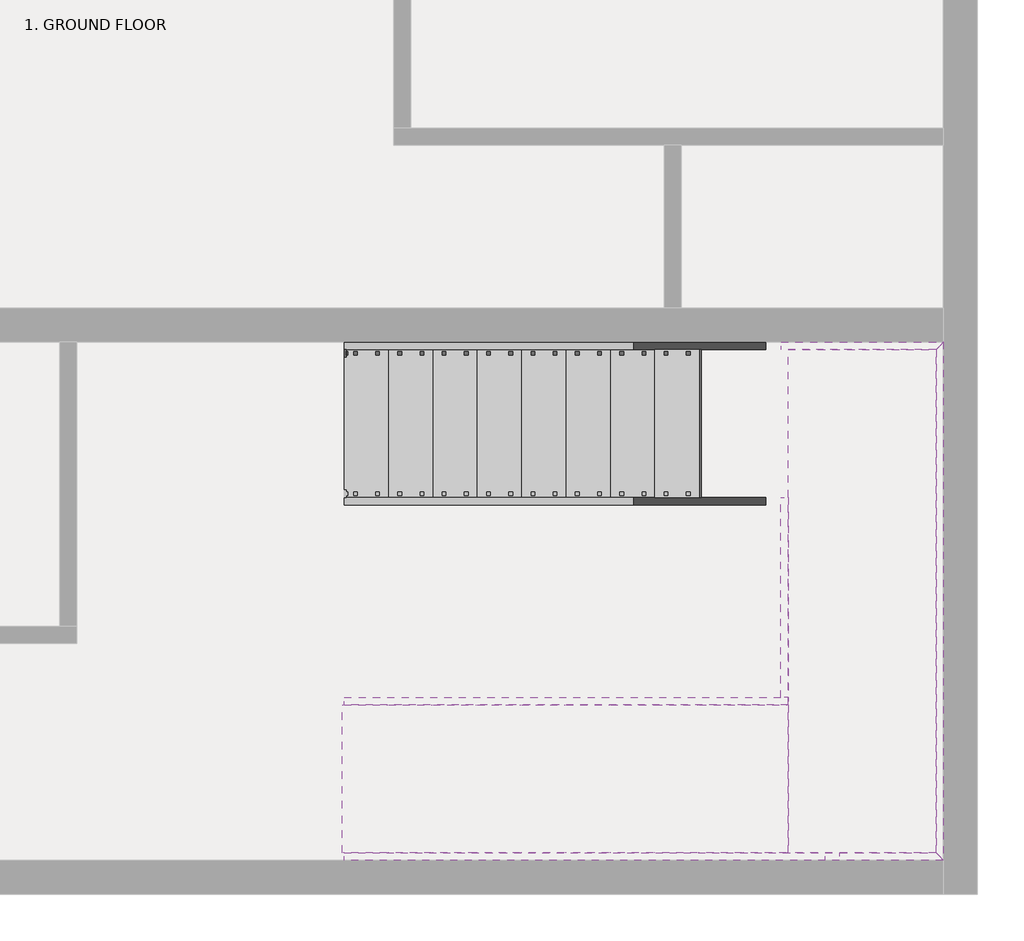
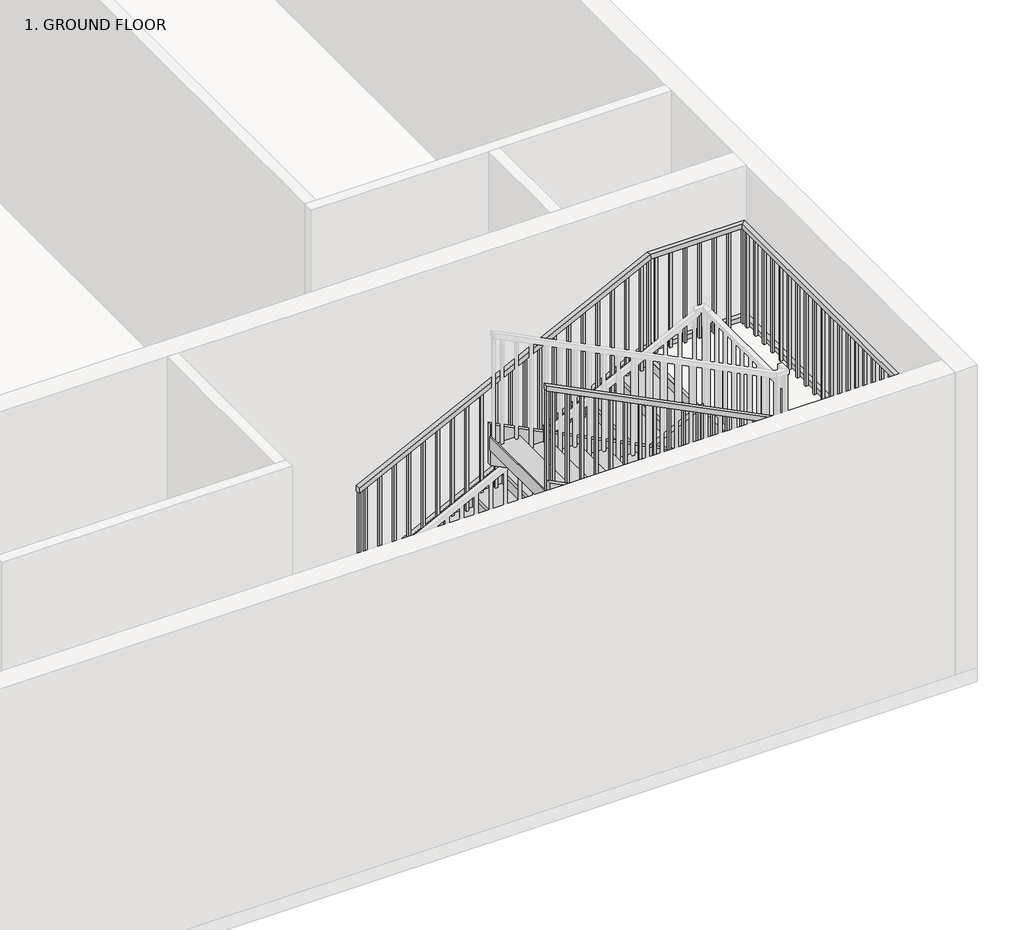
# One storey, part 2 of 2: 8 members, 2 stair flights, 1 railing, 1 slab.
"""IFC4 building model written with IfcOpenShell, lengths in millimetres."""

from ifc_helpers import new_model, si_unit, frame, origin, place, context, project, spatial, polyline, outline, extrude, faceted_brep, transform, mapped, element, save
from components import non_monolithic_landing_146c630b, stair_flight_50mm_tread_13mm_riser_b7d47cc6, stair_flight_50mm_tread_13mm_riser_afbce6aa

model = new_model("IFC4")

# Units and contexts
model_context = context("Model", 3, world=origin())
ifc_project = project(units=[si_unit("LENGTHUNIT", "METRE", prefix="MILLI")], contexts=[model_context])

# Site, building, storey
site = spatial("IfcSite", under=ifc_project)
building = spatial("IfcBuilding", under=site)
storey = spatial("IfcBuildingStorey", under=building, Name="1. GROUND FLOOR", Elevation=0.0)

# Members
placement = place(None, origin())
element("IfcMember", 1, ObjectType="Stringer - 50mm Width", at=placement, inside=storey, context=model_context, shape_type="SweptSolid", body=[
    extrude(outline(polyline([(223.2584972, 1688.8435815), (0.0, 1688.8435815), (0.0, 2136.7537781), (1300.0, 4736.7537781), (1700.0, 4642.3265871), (223.2584972, 1688.8435815)])), frame((0.0, -2974.091395, 0.0), z_axis=(0.0, 1.0, 0.0), x_axis=(0.0, 0.0, 1.0)), (0.0, 0.0, 1.0), 50.0),
])
element("IfcMember", 2, ObjectType="Stringer - 50mm Width", at=placement, inside=storey, context=model_context, shape_type="SweptSolid", body=[
    extrude(outline(polyline([(223.2584972, 1688.8435815), (0.0, 1688.8435815), (0.0, 2136.7537781), (1251.0449017, 4638.8435815), (1698.2584972, 4638.8435815), (223.2584972, 1688.8435815)])), frame((0.0, -4024.091395, 0.0), z_axis=(0.0, 1.0, 0.0), x_axis=(0.0, 0.0, 1.0)), (0.0, 0.0, 1.0), 50.0),
])
element("IfcMember", 3, ObjectType="Stringer - 50mm Width", at=placement, inside=storey, context=model_context, shape_type="SweptSolid", body=[
    extrude(outline(polyline([(1300.0, 4940.9333848), (1700.0, 5035.3605758), (3373.2584972, 1688.8435815), (2926.0449017, 1688.8435815), (1300.0, 4940.9333848)])), frame((0.0, -6426.491395, 0.0), z_axis=(0.0, 1.0, 0.0), x_axis=(0.0, 0.0, 1.0)), (0.0, 0.0, 1.0), 50.0),
])
element("IfcMember", 4, ObjectType="Stringer - 50mm Width", at=placement, inside=storey, context=model_context, shape_type="SweptSolid", body=[
    extrude(outline(polyline([(1426.0449017, 4688.8435815), (1873.2584972, 4688.8435815), (3373.2584972, 1688.8435815), (2926.0449017, 1688.8435815), (1426.0449017, 4688.8435815)])), frame((0.0, -5376.491395, 0.0), z_axis=(0.0, 1.0, 0.0), x_axis=(0.0, 0.0, 1.0)), (0.0, 0.0, 1.0), 50.0),
])
element("IfcMember", 5, ObjectType="Stringer - 50mm Width", at=placement, inside=storey, context=model_context, shape_type="Brep", body=[
    faceted_brep([(5035.3605758, -6376.491395, 1700.0), (5035.3605758, -6426.491395, 1700.0), (5738.8435815, -6426.491395, 1700.0), (5688.8435815, -6376.491395, 1700.0), (4940.9333848, -6376.491395, 1300.0), (5688.8435815, -6376.491395, 1300.0), (4940.9333848, -6426.491395, 1300.0), (5738.8435815, -6426.491395, 1300.0)], [[[0, 1, 2, 3]], [[4, 0, 3, 5]], [[6, 4, 5, 7]], [[1, 6, 7, 2]], [[1, 0, 4, 6]], [[2, 7, 5, 3]]]),
])
element("IfcMember", 6, ObjectType="Stringer - 50mm Width", at=placement, inside=storey, context=model_context, shape_type="SweptSolid", body=[
    extrude(outline(polyline([(5738.8435815, -6426.491395), (5688.8435815, -6376.491395), (5688.8435815, -2974.091395), (5738.8435815, -2924.091395), (5738.8435815, -6426.491395)])), frame((0.0, 0.0, 1300.0), z_axis=(0.0, 0.0, 1.0), x_axis=(1.0, 0.0, 0.0)), (0.0, 0.0, 1.0), 400.0),
])
element("IfcMember", 7, ObjectType="Stringer - 50mm Width", at=placement, inside=storey, context=model_context, shape_type="Brep", body=[
    faceted_brep([(5688.8435815, -2974.091395, 1700.0), (5738.8435815, -2924.091395, 1700.0), (4642.3265871, -2924.091395, 1700.0), (4642.3265871, -2974.091395, 1700.0), (5688.8435815, -2974.091395, 1300.0), (4736.7537781, -2974.091395, 1300.0), (5738.8435815, -2924.091395, 1300.0), (4736.7537781, -2924.091395, 1300.0)], [[[0, 1, 2, 3]], [[4, 0, 3, 5]], [[6, 4, 5, 7]], [[1, 6, 7, 2]], [[1, 0, 4, 6]], [[2, 7, 5, 3]]]),
])
element("IfcMember", 8, ObjectType="Stringer - 50mm Width", at=placement, inside=storey, context=model_context, shape_type="SweptSolid", body=[
    extrude(outline(polyline([(4638.8435815, -3974.091395), (4688.8435815, -3974.091395), (4688.8435815, -5326.491395), (4638.8435815, -5326.491395), (4638.8435815, -3974.091395)])), frame((0.0, 0.0, 1300.0), z_axis=(0.0, 0.0, 1.0), x_axis=(1.0, 0.0, 0.0)), (0.0, 0.0, 1.0), 400.0),
])

# Railing
element("IfcRailing", 9, ObjectType="1100mm", at=placement, inside=storey, context=model_context, shape_type="SolidModel", body=[
    faceted_brep([(1688.8435815, -2974.491395, 1250.0), (1688.8435815, -2974.491395, 1194.0983006), (1688.8435815, -3024.491395, 1194.0983006), (1688.8435815, -3024.491395, 1250.0), (4688.8435815, -2974.491395, 2750.0), (4700.6469803, -2974.491395, 2700.0), (4700.6469803, -3024.491395, 2700.0), (4688.8435815, -3024.491395, 2750.0), (5688.4435815, -2974.491395, 2750.0), (5688.4435815, -2974.491395, 2700.0), (5638.4435815, -3024.491395, 2700.0), (5638.4435815, -3024.491395, 2750.0), (5688.4435815, -6376.091395, 2750.0), (5688.4435815, -6376.091395, 2700.0), (5638.4435815, -6326.091395, 2700.0), (5638.4435815, -6326.091395, 2750.0), (4988.8435815, -6376.091395, 2750.0), (4977.0401826, -6376.091395, 2700.0), (4977.0401826, -6326.091395, 2700.0), (4988.8435815, -6326.091395, 2750.0), (4688.8435815, -6376.091395, 2900.0), (4666.4829017, -6376.091395, 2855.2786405), (4666.4829017, -6326.091395, 2855.2786405), (4688.8435815, -6326.091395, 2900.0), (1688.8435815, -6376.091395, 4400.0), (1688.8435815, -6326.091395, 4400.0), (1688.8435815, -6326.091395, 4344.0983006), (1688.8435815, -6376.091395, 4344.0983006)], [[[0, 1, 2, 3]], [[1, 0, 4, 5]], [[2, 1, 5, 6]], [[3, 2, 6, 7]], [[0, 3, 7, 4]], [[5, 4, 8, 9]], [[6, 5, 9, 10]], [[7, 6, 10, 11]], [[4, 7, 11, 8]], [[9, 8, 12, 13]], [[10, 9, 13, 14]], [[11, 10, 14, 15]], [[8, 11, 15, 12]], [[13, 12, 16, 17]], [[14, 13, 17, 18]], [[15, 14, 18, 19]], [[12, 15, 19, 16]], [[17, 16, 20, 21]], [[18, 17, 21, 22]], [[19, 18, 22, 23]], [[16, 19, 23, 20]], [[24, 25, 26, 27]], [[21, 20, 24, 27]], [[22, 21, 27, 26]], [[23, 22, 26, 25]], [[20, 23, 25, 24]]]),
    extrude(outline(polyline([(4300.3483006, 1776.3435815), (4312.8483006, 1751.3435815), (3150.0, 1751.3435815), (3150.0, 1776.3435815), (4300.3483006, 1776.3435815)])), frame((0.0, -6363.591395, 0.0), z_axis=(0.0, 1.0, 0.0), x_axis=(0.0, 0.0, 1.0)), (0.0, 0.0, 1.0), 25.0),
    extrude(outline(polyline([(4225.3483006, 1926.3435815), (4237.8483006, 1901.3435815), (3150.0, 1901.3435815), (3150.0, 1926.3435815), (4225.3483006, 1926.3435815)])), frame((0.0, -6363.591395, 0.0), z_axis=(0.0, 1.0, 0.0), x_axis=(0.0, 0.0, 1.0)), (0.0, 0.0, 1.0), 25.0),
    extrude(outline(polyline([(4150.3483006, 2076.3435815), (4162.8483006, 2051.3435815), (3000.0, 2051.3435815), (3000.0, 2076.3435815), (4150.3483006, 2076.3435815)])), frame((0.0, -6363.591395, 0.0), z_axis=(0.0, 1.0, 0.0), x_axis=(0.0, 0.0, 1.0)), (0.0, 0.0, 1.0), 25.0),
    extrude(outline(polyline([(4075.3483006, 2226.3435815), (4087.8483006, 2201.3435815), (3000.0, 2201.3435815), (3000.0, 2226.3435815), (4075.3483006, 2226.3435815)])), frame((0.0, -6363.591395, 0.0), z_axis=(0.0, 1.0, 0.0), x_axis=(0.0, 0.0, 1.0)), (0.0, 0.0, 1.0), 25.0),
    extrude(outline(polyline([(4000.3483006, 2376.3435815), (4012.8483006, 2351.3435815), (2850.0, 2351.3435815), (2850.0, 2376.3435815), (4000.3483006, 2376.3435815)])), frame((0.0, -6363.591395, 0.0), z_axis=(0.0, 1.0, 0.0), x_axis=(0.0, 0.0, 1.0)), (0.0, 0.0, 1.0), 25.0),
    extrude(outline(polyline([(3925.3483006, 2526.3435815), (3937.8483006, 2501.3435815), (2850.0, 2501.3435815), (2850.0, 2526.3435815), (3925.3483006, 2526.3435815)])), frame((0.0, -6363.591395, 0.0), z_axis=(0.0, 1.0, 0.0), x_axis=(0.0, 0.0, 1.0)), (0.0, 0.0, 1.0), 25.0),
    extrude(outline(polyline([(3850.3483006, 2676.3435815), (3862.8483006, 2651.3435815), (2700.0, 2651.3435815), (2700.0, 2676.3435815), (3850.3483006, 2676.3435815)])), frame((0.0, -6363.591395, 0.0), z_axis=(0.0, 1.0, 0.0), x_axis=(0.0, 0.0, 1.0)), (0.0, 0.0, 1.0), 25.0),
    extrude(outline(polyline([(3775.3483006, 2826.3435815), (3787.8483006, 2801.3435815), (2700.0, 2801.3435815), (2700.0, 2826.3435815), (3775.3483006, 2826.3435815)])), frame((0.0, -6363.591395, 0.0), z_axis=(0.0, 1.0, 0.0), x_axis=(0.0, 0.0, 1.0)), (0.0, 0.0, 1.0), 25.0),
    extrude(outline(polyline([(3700.3483006, 2976.3435815), (3712.8483006, 2951.3435815), (2550.0, 2951.3435815), (2550.0, 2976.3435815), (3700.3483006, 2976.3435815)])), frame((0.0, -6363.591395, 0.0), z_axis=(0.0, 1.0, 0.0), x_axis=(0.0, 0.0, 1.0)), (0.0, 0.0, 1.0), 25.0),
    extrude(outline(polyline([(3625.3483006, 3126.3435815), (3637.8483006, 3101.3435815), (2550.0, 3101.3435815), (2550.0, 3126.3435815), (3625.3483006, 3126.3435815)])), frame((0.0, -6363.591395, 0.0), z_axis=(0.0, 1.0, 0.0), x_axis=(0.0, 0.0, 1.0)), (0.0, 0.0, 1.0), 25.0),
    extrude(outline(polyline([(3550.3483006, 3276.3435815), (3562.8483006, 3251.3435815), (2400.0, 3251.3435815), (2400.0, 3276.3435815), (3550.3483006, 3276.3435815)])), frame((0.0, -6363.591395, 0.0), z_axis=(0.0, 1.0, 0.0), x_axis=(0.0, 0.0, 1.0)), (0.0, 0.0, 1.0), 25.0),
    extrude(outline(polyline([(3475.3483006, 3426.3435815), (3487.8483006, 3401.3435815), (2400.0, 3401.3435815), (2400.0, 3426.3435815), (3475.3483006, 3426.3435815)])), frame((0.0, -6363.591395, 0.0), z_axis=(0.0, 1.0, 0.0), x_axis=(0.0, 0.0, 1.0)), (0.0, 0.0, 1.0), 25.0),
    extrude(outline(polyline([(3400.3483006, 3576.3435815), (3412.8483006, 3551.3435815), (2250.0, 3551.3435815), (2250.0, 3576.3435815), (3400.3483006, 3576.3435815)])), frame((0.0, -6363.591395, 0.0), z_axis=(0.0, 1.0, 0.0), x_axis=(0.0, 0.0, 1.0)), (0.0, 0.0, 1.0), 25.0),
    extrude(outline(polyline([(3325.3483006, 3726.3435815), (3337.8483006, 3701.3435815), (2250.0, 3701.3435815), (2250.0, 3726.3435815), (3325.3483006, 3726.3435815)])), frame((0.0, -6363.591395, 0.0), z_axis=(0.0, 1.0, 0.0), x_axis=(0.0, 0.0, 1.0)), (0.0, 0.0, 1.0), 25.0),
    extrude(outline(polyline([(3250.3483006, 3876.3435815), (3262.8483006, 3851.3435815), (2100.0, 3851.3435815), (2100.0, 3876.3435815), (3250.3483006, 3876.3435815)])), frame((0.0, -6363.591395, 0.0), z_axis=(0.0, 1.0, 0.0), x_axis=(0.0, 0.0, 1.0)), (0.0, 0.0, 1.0), 25.0),
    extrude(outline(polyline([(3175.3483006, 4026.3435815), (3187.8483006, 4001.3435815), (2100.0, 4001.3435815), (2100.0, 4026.3435815), (3175.3483006, 4026.3435815)])), frame((0.0, -6363.591395, 0.0), z_axis=(0.0, 1.0, 0.0), x_axis=(0.0, 0.0, 1.0)), (0.0, 0.0, 1.0), 25.0),
    extrude(outline(polyline([(3100.3483006, 4176.3435815), (3112.8483006, 4151.3435815), (1950.0, 4151.3435815), (1950.0, 4176.3435815), (3100.3483006, 4176.3435815)])), frame((0.0, -6363.591395, 0.0), z_axis=(0.0, 1.0, 0.0), x_axis=(0.0, 0.0, 1.0)), (0.0, 0.0, 1.0), 25.0),
    extrude(outline(polyline([(3025.3483006, 4326.3435815), (3037.8483006, 4301.3435815), (1950.0, 4301.3435815), (1950.0, 4326.3435815), (3025.3483006, 4326.3435815)])), frame((0.0, -6363.591395, 0.0), z_axis=(0.0, 1.0, 0.0), x_axis=(0.0, 0.0, 1.0)), (0.0, 0.0, 1.0), 25.0),
    extrude(outline(polyline([(2950.3483006, 4476.3435815), (2962.8483006, 4451.3435815), (1800.0, 4451.3435815), (1800.0, 4476.3435815), (2950.3483006, 4476.3435815)])), frame((0.0, -6363.591395, 0.0), z_axis=(0.0, 1.0, 0.0), x_axis=(0.0, 0.0, 1.0)), (0.0, 0.0, 1.0), 25.0),
    extrude(outline(polyline([(2875.3483006, 4626.3435815), (2887.8483006, 4601.3435815), (1800.0, 4601.3435815), (1800.0, 4626.3435815), (2875.3483006, 4626.3435815)])), frame((0.0, -6363.591395, 0.0), z_axis=(0.0, 1.0, 0.0), x_axis=(0.0, 0.0, 1.0)), (0.0, 0.0, 1.0), 25.0),
    extrude(outline(polyline([(2763.0483006, 4850.9435815), (2775.5483006, 4825.9435815), (1650.0, 4825.9435815), (1650.0, 4850.9435815), (2763.0483006, 4850.9435815)])), frame((0.0, -6363.591395, 0.0), z_axis=(0.0, 1.0, 0.0), x_axis=(0.0, 0.0, 1.0)), (0.0, 0.0, 1.0), 25.0),
    extrude(outline(polyline([(2688.0483006, 5000.9435815), (2700.5483006, 4975.9435815), (1650.0, 4975.9435815), (1650.0, 5000.9435815), (2688.0483006, 5000.9435815)])), frame((0.0, -6363.591395, 0.0), z_axis=(0.0, 1.0, 0.0), x_axis=(0.0, 0.0, 1.0)), (0.0, 0.0, 1.0), 25.0),
    extrude(outline(polyline([(5150.9435815, -6363.591395), (5125.9435815, -6363.591395), (5125.9435815, -6338.591395), (5150.9435815, -6338.591395), (5150.9435815, -6363.591395)])), frame((0.0, 0.0, 1650.0), z_axis=(0.0, 0.0, 1.0), x_axis=(1.0, 0.0, 0.0)), (0.0, 0.0, 1.0), 1050.0),
    extrude(outline(polyline([(5300.9435815, -6363.591395), (5275.9435815, -6363.591395), (5275.9435815, -6338.591395), (5300.9435815, -6338.591395), (5300.9435815, -6363.591395)])), frame((0.0, 0.0, 1650.0), z_axis=(0.0, 0.0, 1.0), x_axis=(1.0, 0.0, 0.0)), (0.0, 0.0, 1.0), 1050.0),
    extrude(outline(polyline([(5450.9435815, -6363.591395), (5425.9435815, -6363.591395), (5425.9435815, -6338.591395), (5450.9435815, -6338.591395), (5450.9435815, -6363.591395)])), frame((0.0, 0.0, 1650.0), z_axis=(0.0, 0.0, 1.0), x_axis=(1.0, 0.0, 0.0)), (0.0, 0.0, 1.0), 1050.0),
    extrude(outline(polyline([(5600.9435815, -6363.591395), (5575.9435815, -6363.591395), (5575.9435815, -6338.591395), (5600.9435815, -6338.591395), (5600.9435815, -6363.591395)])), frame((0.0, 0.0, 1650.0), z_axis=(0.0, 0.0, 1.0), x_axis=(1.0, 0.0, 0.0)), (0.0, 0.0, 1.0), 1050.0),
    extrude(outline(polyline([(5675.9435815, -6211.991395), (5675.9435815, -6236.991395), (5650.9435815, -6236.991395), (5650.9435815, -6211.991395), (5675.9435815, -6211.991395)])), frame((0.0, 0.0, 1650.0), z_axis=(0.0, 0.0, 1.0), x_axis=(1.0, 0.0, 0.0)), (0.0, 0.0, 1.0), 1050.0),
    extrude(outline(polyline([(5675.9435815, -6061.991395), (5675.9435815, -6086.991395), (5650.9435815, -6086.991395), (5650.9435815, -6061.991395), (5675.9435815, -6061.991395)])), frame((0.0, 0.0, 1650.0), z_axis=(0.0, 0.0, 1.0), x_axis=(1.0, 0.0, 0.0)), (0.0, 0.0, 1.0), 1050.0),
    extrude(outline(polyline([(5675.9435815, -5911.991395), (5675.9435815, -5936.991395), (5650.9435815, -5936.991395), (5650.9435815, -5911.991395), (5675.9435815, -5911.991395)])), frame((0.0, 0.0, 1650.0), z_axis=(0.0, 0.0, 1.0), x_axis=(1.0, 0.0, 0.0)), (0.0, 0.0, 1.0), 1050.0),
    extrude(outline(polyline([(5675.9435815, -5761.991395), (5675.9435815, -5786.991395), (5650.9435815, -5786.991395), (5650.9435815, -5761.991395), (5675.9435815, -5761.991395)])), frame((0.0, 0.0, 1650.0), z_axis=(0.0, 0.0, 1.0), x_axis=(1.0, 0.0, 0.0)), (0.0, 0.0, 1.0), 1050.0),
    extrude(outline(polyline([(5675.9435815, -5611.991395), (5675.9435815, -5636.991395), (5650.9435815, -5636.991395), (5650.9435815, -5611.991395), (5675.9435815, -5611.991395)])), frame((0.0, 0.0, 1650.0), z_axis=(0.0, 0.0, 1.0), x_axis=(1.0, 0.0, 0.0)), (0.0, 0.0, 1.0), 1050.0),
    extrude(outline(polyline([(5675.9435815, -5461.991395), (5675.9435815, -5486.991395), (5650.9435815, -5486.991395), (5650.9435815, -5461.991395), (5675.9435815, -5461.991395)])), frame((0.0, 0.0, 1650.0), z_axis=(0.0, 0.0, 1.0), x_axis=(1.0, 0.0, 0.0)), (0.0, 0.0, 1.0), 1050.0),
    extrude(outline(polyline([(5675.9435815, -5311.991395), (5675.9435815, -5336.991395), (5650.9435815, -5336.991395), (5650.9435815, -5311.991395), (5675.9435815, -5311.991395)])), frame((0.0, 0.0, 1650.0), z_axis=(0.0, 0.0, 1.0), x_axis=(1.0, 0.0, 0.0)), (0.0, 0.0, 1.0), 1050.0),
    extrude(outline(polyline([(5675.9435815, -5161.991395), (5675.9435815, -5186.991395), (5650.9435815, -5186.991395), (5650.9435815, -5161.991395), (5675.9435815, -5161.991395)])), frame((0.0, 0.0, 1650.0), z_axis=(0.0, 0.0, 1.0), x_axis=(1.0, 0.0, 0.0)), (0.0, 0.0, 1.0), 1050.0),
    extrude(outline(polyline([(5675.9435815, -5011.991395), (5675.9435815, -5036.991395), (5650.9435815, -5036.991395), (5650.9435815, -5011.991395), (5675.9435815, -5011.991395)])), frame((0.0, 0.0, 1650.0), z_axis=(0.0, 0.0, 1.0), x_axis=(1.0, 0.0, 0.0)), (0.0, 0.0, 1.0), 1050.0),
    extrude(outline(polyline([(5675.9435815, -4861.991395), (5675.9435815, -4886.991395), (5650.9435815, -4886.991395), (5650.9435815, -4861.991395), (5675.9435815, -4861.991395)])), frame((0.0, 0.0, 1650.0), z_axis=(0.0, 0.0, 1.0), x_axis=(1.0, 0.0, 0.0)), (0.0, 0.0, 1.0), 1050.0),
    extrude(outline(polyline([(5675.9435815, -4711.991395), (5675.9435815, -4736.991395), (5650.9435815, -4736.991395), (5650.9435815, -4711.991395), (5675.9435815, -4711.991395)])), frame((0.0, 0.0, 1650.0), z_axis=(0.0, 0.0, 1.0), x_axis=(1.0, 0.0, 0.0)), (0.0, 0.0, 1.0), 1050.0),
    extrude(outline(polyline([(5675.9435815, -4561.991395), (5675.9435815, -4586.991395), (5650.9435815, -4586.991395), (5650.9435815, -4561.991395), (5675.9435815, -4561.991395)])), frame((0.0, 0.0, 1650.0), z_axis=(0.0, 0.0, 1.0), x_axis=(1.0, 0.0, 0.0)), (0.0, 0.0, 1.0), 1050.0),
    extrude(outline(polyline([(5675.9435815, -4411.991395), (5675.9435815, -4436.991395), (5650.9435815, -4436.991395), (5650.9435815, -4411.991395), (5675.9435815, -4411.991395)])), frame((0.0, 0.0, 1650.0), z_axis=(0.0, 0.0, 1.0), x_axis=(1.0, 0.0, 0.0)), (0.0, 0.0, 1.0), 1050.0),
    extrude(outline(polyline([(5675.9435815, -4261.991395), (5675.9435815, -4286.991395), (5650.9435815, -4286.991395), (5650.9435815, -4261.991395), (5675.9435815, -4261.991395)])), frame((0.0, 0.0, 1650.0), z_axis=(0.0, 0.0, 1.0), x_axis=(1.0, 0.0, 0.0)), (0.0, 0.0, 1.0), 1050.0),
    extrude(outline(polyline([(5675.9435815, -4111.991395), (5675.9435815, -4136.991395), (5650.9435815, -4136.991395), (5650.9435815, -4111.991395), (5675.9435815, -4111.991395)])), frame((0.0, 0.0, 1650.0), z_axis=(0.0, 0.0, 1.0), x_axis=(1.0, 0.0, 0.0)), (0.0, 0.0, 1.0), 1050.0),
    extrude(outline(polyline([(5675.9435815, -3961.991395), (5675.9435815, -3986.991395), (5650.9435815, -3986.991395), (5650.9435815, -3961.991395), (5675.9435815, -3961.991395)])), frame((0.0, 0.0, 1650.0), z_axis=(0.0, 0.0, 1.0), x_axis=(1.0, 0.0, 0.0)), (0.0, 0.0, 1.0), 1050.0),
    extrude(outline(polyline([(5675.9435815, -3811.991395), (5675.9435815, -3836.991395), (5650.9435815, -3836.991395), (5650.9435815, -3811.991395), (5675.9435815, -3811.991395)])), frame((0.0, 0.0, 1650.0), z_axis=(0.0, 0.0, 1.0), x_axis=(1.0, 0.0, 0.0)), (0.0, 0.0, 1.0), 1050.0),
    extrude(outline(polyline([(5675.9435815, -3661.991395), (5675.9435815, -3686.991395), (5650.9435815, -3686.991395), (5650.9435815, -3661.991395), (5675.9435815, -3661.991395)])), frame((0.0, 0.0, 1650.0), z_axis=(0.0, 0.0, 1.0), x_axis=(1.0, 0.0, 0.0)), (0.0, 0.0, 1.0), 1050.0),
    extrude(outline(polyline([(5675.9435815, -3511.991395), (5675.9435815, -3536.991395), (5650.9435815, -3536.991395), (5650.9435815, -3511.991395), (5675.9435815, -3511.991395)])), frame((0.0, 0.0, 1650.0), z_axis=(0.0, 0.0, 1.0), x_axis=(1.0, 0.0, 0.0)), (0.0, 0.0, 1.0), 1050.0),
    extrude(outline(polyline([(5675.9435815, -3361.991395), (5675.9435815, -3386.991395), (5650.9435815, -3386.991395), (5650.9435815, -3361.991395), (5675.9435815, -3361.991395)])), frame((0.0, 0.0, 1650.0), z_axis=(0.0, 0.0, 1.0), x_axis=(1.0, 0.0, 0.0)), (0.0, 0.0, 1.0), 1050.0),
    extrude(outline(polyline([(5675.9435815, -3211.991395), (5675.9435815, -3236.991395), (5650.9435815, -3236.991395), (5650.9435815, -3211.991395), (5675.9435815, -3211.991395)])), frame((0.0, 0.0, 1650.0), z_axis=(0.0, 0.0, 1.0), x_axis=(1.0, 0.0, 0.0)), (0.0, 0.0, 1.0), 1050.0),
    extrude(outline(polyline([(5675.9435815, -3061.991395), (5675.9435815, -3086.991395), (5650.9435815, -3086.991395), (5650.9435815, -3061.991395), (5675.9435815, -3061.991395)])), frame((0.0, 0.0, 1650.0), z_axis=(0.0, 0.0, 1.0), x_axis=(1.0, 0.0, 0.0)), (0.0, 0.0, 1.0), 1050.0),
    extrude(outline(polyline([(5501.3435815, -2986.991395), (5526.3435815, -2986.991395), (5526.3435815, -3011.991395), (5501.3435815, -3011.991395), (5501.3435815, -2986.991395)])), frame((0.0, 0.0, 1650.0), z_axis=(0.0, 0.0, 1.0), x_axis=(1.0, 0.0, 0.0)), (0.0, 0.0, 1.0), 1050.0),
    extrude(outline(polyline([(5351.3435815, -2986.991395), (5376.3435815, -2986.991395), (5376.3435815, -3011.991395), (5351.3435815, -3011.991395), (5351.3435815, -2986.991395)])), frame((0.0, 0.0, 1650.0), z_axis=(0.0, 0.0, 1.0), x_axis=(1.0, 0.0, 0.0)), (0.0, 0.0, 1.0), 1050.0),
    extrude(outline(polyline([(5201.3435815, -2986.991395), (5226.3435815, -2986.991395), (5226.3435815, -3011.991395), (5201.3435815, -3011.991395), (5201.3435815, -2986.991395)])), frame((0.0, 0.0, 1650.0), z_axis=(0.0, 0.0, 1.0), x_axis=(1.0, 0.0, 0.0)), (0.0, 0.0, 1.0), 1050.0),
    extrude(outline(polyline([(5051.3435815, -2986.991395), (5076.3435815, -2986.991395), (5076.3435815, -3011.991395), (5051.3435815, -3011.991395), (5051.3435815, -2986.991395)])), frame((0.0, 0.0, 1650.0), z_axis=(0.0, 0.0, 1.0), x_axis=(1.0, 0.0, 0.0)), (0.0, 0.0, 1.0), 1050.0),
    extrude(outline(polyline([(4901.3435815, -2986.991395), (4926.3435815, -2986.991395), (4926.3435815, -3011.991395), (4901.3435815, -3011.991395), (4901.3435815, -2986.991395)])), frame((0.0, 0.0, 1650.0), z_axis=(0.0, 0.0, 1.0), x_axis=(1.0, 0.0, 0.0)), (0.0, 0.0, 1.0), 1050.0),
    extrude(outline(polyline([(4751.3435815, -2986.991395), (4776.3435815, -2986.991395), (4776.3435815, -3011.991395), (4751.3435815, -3011.991395), (4751.3435815, -2986.991395)])), frame((0.0, 0.0, 1650.0), z_axis=(0.0, 0.0, 1.0), x_axis=(1.0, 0.0, 0.0)), (0.0, 0.0, 1.0), 1050.0),
    extrude(outline(polyline([(1500.0, 4601.3435815), (1500.0, 4626.3435815), (2662.8483006, 4626.3435815), (2650.3483006, 4601.3435815), (1500.0, 4601.3435815)])), frame((0.0, -3011.991395, 0.0), z_axis=(0.0, 1.0, 0.0), x_axis=(0.0, 0.0, 1.0)), (0.0, 0.0, 1.0), 25.0),
    extrude(outline(polyline([(1500.0, 4451.3435815), (1500.0, 4476.3435815), (2587.8483006, 4476.3435815), (2575.3483006, 4451.3435815), (1500.0, 4451.3435815)])), frame((0.0, -3011.991395, 0.0), z_axis=(0.0, 1.0, 0.0), x_axis=(0.0, 0.0, 1.0)), (0.0, 0.0, 1.0), 25.0),
    extrude(outline(polyline([(1350.0, 4301.3435815), (1350.0, 4326.3435815), (2512.8483006, 4326.3435815), (2500.3483006, 4301.3435815), (1350.0, 4301.3435815)])), frame((0.0, -3011.991395, 0.0), z_axis=(0.0, 1.0, 0.0), x_axis=(0.0, 0.0, 1.0)), (0.0, 0.0, 1.0), 25.0),
    extrude(outline(polyline([(1350.0, 4151.3435815), (1350.0, 4176.3435815), (2437.8483006, 4176.3435815), (2425.3483006, 4151.3435815), (1350.0, 4151.3435815)])), frame((0.0, -3011.991395, 0.0), z_axis=(0.0, 1.0, 0.0), x_axis=(0.0, 0.0, 1.0)), (0.0, 0.0, 1.0), 25.0),
    extrude(outline(polyline([(1200.0, 4001.3435815), (1200.0, 4026.3435815), (2362.8483006, 4026.3435815), (2350.3483006, 4001.3435815), (1200.0, 4001.3435815)])), frame((0.0, -3011.991395, 0.0), z_axis=(0.0, 1.0, 0.0), x_axis=(0.0, 0.0, 1.0)), (0.0, 0.0, 1.0), 25.0),
    extrude(outline(polyline([(1200.0, 3851.3435815), (1200.0, 3876.3435815), (2287.8483006, 3876.3435815), (2275.3483006, 3851.3435815), (1200.0, 3851.3435815)])), frame((0.0, -3011.991395, 0.0), z_axis=(0.0, 1.0, 0.0), x_axis=(0.0, 0.0, 1.0)), (0.0, 0.0, 1.0), 25.0),
    extrude(outline(polyline([(1050.0, 3701.3435815), (1050.0, 3726.3435815), (2212.8483006, 3726.3435815), (2200.3483006, 3701.3435815), (1050.0, 3701.3435815)])), frame((0.0, -3011.991395, 0.0), z_axis=(0.0, 1.0, 0.0), x_axis=(0.0, 0.0, 1.0)), (0.0, 0.0, 1.0), 25.0),
    extrude(outline(polyline([(1050.0, 3551.3435815), (1050.0, 3576.3435815), (2137.8483006, 3576.3435815), (2125.3483006, 3551.3435815), (1050.0, 3551.3435815)])), frame((0.0, -3011.991395, 0.0), z_axis=(0.0, 1.0, 0.0), x_axis=(0.0, 0.0, 1.0)), (0.0, 0.0, 1.0), 25.0),
    extrude(outline(polyline([(900.0, 3401.3435815), (900.0, 3426.3435815), (2062.8483006, 3426.3435815), (2050.3483006, 3401.3435815), (900.0, 3401.3435815)])), frame((0.0, -3011.991395, 0.0), z_axis=(0.0, 1.0, 0.0), x_axis=(0.0, 0.0, 1.0)), (0.0, 0.0, 1.0), 25.0),
    extrude(outline(polyline([(900.0, 3251.3435815), (900.0, 3276.3435815), (1987.8483006, 3276.3435815), (1975.3483006, 3251.3435815), (900.0, 3251.3435815)])), frame((0.0, -3011.991395, 0.0), z_axis=(0.0, 1.0, 0.0), x_axis=(0.0, 0.0, 1.0)), (0.0, 0.0, 1.0), 25.0),
    extrude(outline(polyline([(750.0, 3101.3435815), (750.0, 3126.3435815), (1912.8483006, 3126.3435815), (1900.3483006, 3101.3435815), (750.0, 3101.3435815)])), frame((0.0, -3011.991395, 0.0), z_axis=(0.0, 1.0, 0.0), x_axis=(0.0, 0.0, 1.0)), (0.0, 0.0, 1.0), 25.0),
    extrude(outline(polyline([(750.0, 2951.3435815), (750.0, 2976.3435815), (1837.8483006, 2976.3435815), (1825.3483006, 2951.3435815), (750.0, 2951.3435815)])), frame((0.0, -3011.991395, 0.0), z_axis=(0.0, 1.0, 0.0), x_axis=(0.0, 0.0, 1.0)), (0.0, 0.0, 1.0), 25.0),
    extrude(outline(polyline([(600.0, 2801.3435815), (600.0, 2826.3435815), (1762.8483006, 2826.3435815), (1750.3483006, 2801.3435815), (600.0, 2801.3435815)])), frame((0.0, -3011.991395, 0.0), z_axis=(0.0, 1.0, 0.0), x_axis=(0.0, 0.0, 1.0)), (0.0, 0.0, 1.0), 25.0),
    extrude(outline(polyline([(600.0, 2651.3435815), (600.0, 2676.3435815), (1687.8483006, 2676.3435815), (1675.3483006, 2651.3435815), (600.0, 2651.3435815)])), frame((0.0, -3011.991395, 0.0), z_axis=(0.0, 1.0, 0.0), x_axis=(0.0, 0.0, 1.0)), (0.0, 0.0, 1.0), 25.0),
    extrude(outline(polyline([(450.0, 2501.3435815), (450.0, 2526.3435815), (1612.8483006, 2526.3435815), (1600.3483006, 2501.3435815), (450.0, 2501.3435815)])), frame((0.0, -3011.991395, 0.0), z_axis=(0.0, 1.0, 0.0), x_axis=(0.0, 0.0, 1.0)), (0.0, 0.0, 1.0), 25.0),
    extrude(outline(polyline([(450.0, 2351.3435815), (450.0, 2376.3435815), (1537.8483006, 2376.3435815), (1525.3483006, 2351.3435815), (450.0, 2351.3435815)])), frame((0.0, -3011.991395, 0.0), z_axis=(0.0, 1.0, 0.0), x_axis=(0.0, 0.0, 1.0)), (0.0, 0.0, 1.0), 25.0),
    extrude(outline(polyline([(300.0, 2201.3435815), (300.0, 2226.3435815), (1462.8483006, 2226.3435815), (1450.3483006, 2201.3435815), (300.0, 2201.3435815)])), frame((0.0, -3011.991395, 0.0), z_axis=(0.0, 1.0, 0.0), x_axis=(0.0, 0.0, 1.0)), (0.0, 0.0, 1.0), 25.0),
    extrude(outline(polyline([(300.0, 2051.3435815), (300.0, 2076.3435815), (1387.8483006, 2076.3435815), (1375.3483006, 2051.3435815), (300.0, 2051.3435815)])), frame((0.0, -3011.991395, 0.0), z_axis=(0.0, 1.0, 0.0), x_axis=(0.0, 0.0, 1.0)), (0.0, 0.0, 1.0), 25.0),
    extrude(outline(polyline([(150.0, 1901.3435815), (150.0, 1926.3435815), (1312.8483006, 1926.3435815), (1300.3483006, 1901.3435815), (150.0, 1901.3435815)])), frame((0.0, -3011.991395, 0.0), z_axis=(0.0, 1.0, 0.0), x_axis=(0.0, 0.0, 1.0)), (0.0, 0.0, 1.0), 25.0),
    extrude(outline(polyline([(150.0, 1751.3435815), (150.0, 1776.3435815), (1237.8483006, 1776.3435815), (1225.3483006, 1751.3435815), (150.0, 1751.3435815)])), frame((0.0, -3011.991395, 0.0), z_axis=(0.0, 1.0, 0.0), x_axis=(0.0, 0.0, 1.0)), (0.0, 0.0, 1.0), 25.0),
    extrude(outline(polyline([(2837.8483006, 4701.3435815), (2850.3483006, 4676.3435815), (1650.0, 4676.3435815), (1650.0, 4701.3435815), (2837.8483006, 4701.3435815)])), frame((0.0, -6363.591395, 0.0), z_axis=(0.0, 1.0, 0.0), x_axis=(0.0, 0.0, 1.0)), (0.0, 0.0, 1.0), 25.0),
    extrude(outline(polyline([(5675.9435815, -6338.591395), (5675.9435815, -6363.591395), (5650.9435815, -6363.591395), (5650.9435815, -6338.591395), (5675.9435815, -6338.591395)])), frame((0.0, 0.0, 1650.0), z_axis=(0.0, 0.0, 1.0), x_axis=(1.0, 0.0, 0.0)), (0.0, 0.0, 1.0), 1050.0),
    extrude(outline(polyline([(5650.9435815, -2986.991395), (5675.9435815, -2986.991395), (5675.9435815, -3011.991395), (5650.9435815, -3011.991395), (5650.9435815, -2986.991395)])), frame((0.0, 0.0, 1650.0), z_axis=(0.0, 0.0, 1.0), x_axis=(1.0, 0.0, 0.0)), (0.0, 0.0, 1.0), 1050.0),
    extrude(outline(polyline([(1650.0, 4676.3435815), (1650.0, 4701.3435815), (2700.3483006, 4701.3435815), (2687.8483006, 4676.3435815), (1650.0, 4676.3435815)])), frame((0.0, -3011.991395, 0.0), z_axis=(0.0, 1.0, 0.0), x_axis=(0.0, 0.0, 1.0)), (0.0, 0.0, 1.0), 25.0),
    extrude(outline(polyline([(4331.5983006, 1713.8435815), (4344.0983006, 1688.8435815), (3150.0, 1688.8435815), (3150.0, 1713.8435815), (4331.5983006, 1713.8435815)])), frame((0.0, -6363.591395, 0.0), z_axis=(0.0, 1.0, 0.0), x_axis=(0.0, 0.0, 1.0)), (0.0, 0.0, 1.0), 25.0),
    extrude(outline(polyline([(150.0, 1688.8435815), (150.0, 1713.8435815), (1206.5983006, 1713.8435815), (1194.0983006, 1688.8435815), (150.0, 1688.8435815)])), frame((0.0, -3011.991395, 0.0), z_axis=(0.0, 1.0, 0.0), x_axis=(0.0, 0.0, 1.0)), (0.0, 0.0, 1.0), 25.0),
])

# Slab
non_monolithic_landing_shape = non_monolithic_landing_146c630b(model_context)
element("IfcSlab", 10, ObjectType="Non-Monolithic Landing", at=placement, inside=storey, context=model_context, shape_type="MappedRepresentation", body=[
    mapped(non_monolithic_landing_shape, transform((0.0, 0.0, 0.0), x_axis=(1.0, 0.0, 0.0), y_axis=(0.0, 1.0, 0.0), z_axis=(0.0, 0.0, 1.0))),
])

# Stair flights
stair_flight_50mm_tread_13mm_riser_shape = stair_flight_50mm_tread_13mm_riser_b7d47cc6(model_context)
element("IfcStairFlight", 11, ObjectType="50mm Tread 13mm Riser", at=placement, inside=storey, context=model_context, shape_type="MappedRepresentation", body=[
    mapped(stair_flight_50mm_tread_13mm_riser_shape, transform((0.0, 0.0, 0.0), x_axis=(1.0, 0.0, 0.0), y_axis=(0.0, 1.0, 0.0), z_axis=(0.0, 0.0, 1.0))),
])
stair_flight_50mm_tread_13mm_riser_2_shape = stair_flight_50mm_tread_13mm_riser_afbce6aa(model_context)
element("IfcStairFlight", 12, ObjectType="50mm Tread 13mm Riser", at=placement, inside=storey, context=model_context, shape_type="MappedRepresentation", body=[
    mapped(stair_flight_50mm_tread_13mm_riser_2_shape, transform((0.0, 0.0, 0.0), x_axis=(1.0, 0.0, 0.0), y_axis=(0.0, 1.0, 0.0), z_axis=(0.0, 0.0, 1.0))),
])

save(model, "model.ifc")

# Revit data of these elements
# Type "1100mm"
#   built-in parameter 1008612 = 0.019685 (stored number, unit not read)
#   built-in parameter 1008611 = 0.019685 (stored number, unit not read)
#   built-in parameter 1008609 = 0.902231 (stored number, unit not read)
#   built-in parameter 1008604 = 0.19685 (stored number, unit not read)
#   built-in parameter 1008603 = 0.164042 (stored number, unit not read)
#   Railing Height = 1100 mm
#   built-in parameter 1008630 = 2
#   built-in parameter 1008610 = 2
#   built-in parameter 1008608 = 1
#   built-in parameter 1008618 = M_Baluster - Square : 25mm
# Elements 1, 2, 3, 4, 5, 6, 7, 8 (IfcMember, "Stringer - 50mm Width")
#   Phase Created = New Construction
# Element 9 (IfcRailing, "1100mm")
#   Phase Created = New Construction
# Element 10 (IfcSlab, "Non-Monolithic Landing")
#   Phase Created = New Construction
# Elements 11, 12 (IfcStairFlight, "50mm Tread 13mm Riser")
#   Phase Created = New Construction
